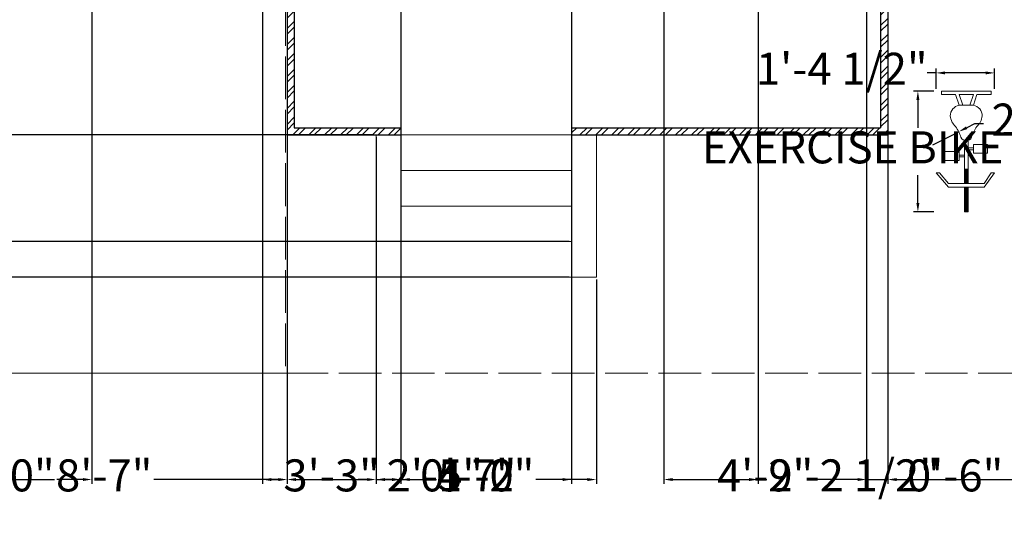
# Model space of a CAD drawing. Units: inches. Extents: x 9689 to 10369, y 10965 to 11626.
# Tile 2 of 11: x 9830 to 10107, y 10965 to 11108. Entities that reach past the tile are written whole.
import ezdxf

# ---------------------------------------------------------------- set-up
doc = ezdxf.new("R2010")
doc.units = ezdxf.units.IN
doc.linetypes.add('ACAD_ISO02W100', pattern=[15, 12, -3])
for name, color, linetype, lineweight in [('A-ANNO-DIMS', 2, 'Continuous', 18), ('A-EQPM', 8, 'Continuous', 18), ('A-FLOR', 7, 'Continuous', 25), ('A-FLOR-PATT', 252, 'Continuous', 13), ('A-FLOR-STRS', 7, 'Continuous', 18), ('C-PARK', 7, 'ACAD_ISO02W100', 18)]:
    doc.layers.add(name, color=color, linetype=linetype, lineweight=lineweight)
doc.styles.get("Standard").update_dxf_attribs({"font": 'arial.ttf'})
doc.dimstyles.new('ISO-25', dxfattribs={"dimtxt": 9, "dimasz": 2.5, "dimexe": 1.25, "dimexo": 0.625, "dimgap": 2, "dimtad": 0, "dimtih": 1, "dimtoh": 1, "dimdec": 1, "dimlunit": 4, "dimtxsty": 'Standard', "dimcen": 2.5, "dimadec": 0, "dimazin": 0, "dimtfac": 0.5, "dimtdec": 1, "dimtmove": 0, "dimatfit": 3, "dimfxl": 1, "dimarcsym": 0})

# ---------------------------------------------------------------- blocks, each defined once
blk = doc.blocks.new('Exercise Bike')
for p, q in [((-0.75, 10), (-0.75, 17)), ((-0.75, 17), (0.25, 17)), ((-0.5, 17), (-0.5, 9.9929)), ((-0.25, 10), (-0.25, 17)), ((0, 17), (0, 9.9929)), ((0.25, 17), (0.25, 10)), ((-5.25, 10), (-8.25, 6)), ((-7.25, 6), (-5.25, 9)), ((-0.75, 10), (-5.25, 10)), ((-5.25, 9), (4.75, 9)), ((4.75, 10), (-0.75, 10)), ((-0.75, 5), (-0.75, 9)), ((-0.5, 8.9396), (-0.5, 5)), ((-0.25, 5), (-0.25, 9)), ((0, 8.9396), (0, 5)), ((0.25, 9), (0.25, 5)), ((8.25, 6), (4.75, 10)), ((4.75, 9), (7.25, 6)), ((-8.25, 6), (-7.25, 6)), ((7.25, 6), (8.25, 6)), ((-0.75, -3.0635), (-0.75, 5)), ((-0.75, 5), (0.25, 5)), ((0.25, 5), (0.25, -3.0635)), ((-6.25, -2), (-6.25, 0.5)), ((-2.25, 0.5), (-6.25, 0.5)), ((-2.25, -0.5), (-2.25, 0.5)), ((0.25, 1.5), (1.75, 1.5)), ((0.25, 1), (1.75, 1)), ((1.75, 2.5), (5.75, 2.5)), ((1.75, 1.5), (1.75, 2.5)), ((1.75, 1.5), (1.75, 0)), ((1.75, 0), (5.75, 0)), ((5.75, 2.5), (5.75, 0)), ((-2.25, -2), (-6.25, -2)), ((-2.25, -0.5), (-0.75, -0.5)), ((-2.25, -1), (-2.25, -0.5)), ((-2.25, -1), (-2.25, -2)), ((-0.75, -1), (-2.25, -1)), ((-2.25, -13), (-3.25, -16)), ((-2.25, -16), (-1.25, -13)), ((-2.25, -13), (1.75, -13)), ((0.75, -13), (1.75, -16)), ((1.75, -13), (2.75, -16)), ((-7.25, -16), (-7.25, -17)), ((-4.75, -16), (-7.25, -16)), ((-3.25, -16), (-4.75, -16)), ((1.75, -16), (-2.25, -16)), ((6.75, -16), (2.75, -16)), ((6.75, -17), (6.75, -16)), ((-7.25, -17), (6.75, -17))]:
    blk.add_line(p, q)
for centre, radius, start, end in [((-9.6692, -1.9154), 8.1889, 321.6175, 345.2525), ((-0.25, -4.625), 1.625, 22.61987, 157.3801), ((9.1691, -1.9154), 8.1889, 194.7476, 218.3825), ((0.1685, -10.5843), 4.9531, 133.6443, 173.2256), ((-0.6686, -10.5843), 4.9531, 6.774486, 46.35562), ((-1.7006, -10.0005), 3.0494, 179.9906, 259.6205), ((1.2006, -10.0005), 3.0494, 280.3795, 0.009389)]:
    blk.add_arc(centre, radius, start, end)
blk = doc.blocks.new('*D62')
at = {"layer": 'A-ANNO-DIMS', "color": 0, "lineweight": -2, "transparency": 16777216}
for p, q in [((10087.02, 11087.95), (10081.3, 11087.95)), ((10082.55, 11085.45), (10082.55, 11077.6)), ((10082.55, 11056.45), (10082.55, 11064.29)), ((10087.02, 11053.95), (10081.3, 11053.95))]:
    blk.add_line(p, q, dxfattribs=at)
at = {"layer": 'A-ANNO-DIMS', "color": 0, "transparency": 16777216}
for points in [[(10082.13, 11085.45), (10082.96, 11085.45), (10082.55, 11087.95)], [(10082.13, 11056.45), (10082.96, 11056.45), (10082.55, 11053.95)]]:
    blk.add_solid(points, dxfattribs=at)
at = {"layer": 'Defpoints', "color": 0, "transparency": 16777216}
for p in [(10087.65, 11087.95), (10082.55, 11053.95), (10087.65, 11053.95)]:
    blk.add_point(p, dxfattribs=at)
at = {"layer": 'A-ANNO-DIMS', "color": 0, "transparency": 16777216, "insert": (10082.55, 11070.95), "char_height": 9, "attachment_point": 5}
blk.add_mtext('EXERCISE BIKE 2\'-10"', dxfattribs=at)
blk = doc.blocks.new('*D63')
at = {"layer": 'A-ANNO-DIMS', "color": 0, "lineweight": -2, "transparency": 16777216}
for p, q in [((10087.65, 11093.05), (10085.15, 11093.05)), ((10087.65, 11088.57), (10087.65, 11094.3)), ((10101.65, 11093.05), (10090.15, 11093.05)), ((10104.15, 11088.57), (10104.15, 11094.3))]:
    blk.add_line(p, q, dxfattribs=at)
at = {"layer": 'A-ANNO-DIMS', "color": 0, "transparency": 16777216}
for points in [[(10090.15, 11093.46), (10090.15, 11092.63), (10087.65, 11093.05)], [(10101.65, 11093.46), (10101.65, 11092.63), (10104.15, 11093.05)]]:
    blk.add_solid(points, dxfattribs=at)
at = {"layer": 'Defpoints', "color": 0, "transparency": 16777216}
for p in [(10087.65, 11093.05), (10087.65, 11087.95), (10104.15, 11087.95)]:
    blk.add_point(p, dxfattribs=at)
at = {"layer": 'A-ANNO-DIMS', "color": 0, "transparency": 16777216, "insert": (10061.12, 11093.05), "char_height": 9, "attachment_point": 5}
blk.add_mtext('1\'-4 1/2"', dxfattribs=at)
blk = doc.blocks.new('*D67')
at = {"layer": 'A-ANNO-DIMS', "color": 0, "lineweight": -2, "transparency": 16777216}
for p, q in [((9802.06, 11157.01), (9802.06, 10977.48)), ((9905.06, 11157.01), (9905.06, 10977.48)), ((9804.56, 10978.73), (9839.59, 10978.73)), ((9902.56, 10978.73), (9867.53, 10978.73))]:
    blk.add_line(p, q, dxfattribs=at)
at = {"layer": 'A-ANNO-DIMS', "color": 0, "transparency": 16777216}
for points in [[(9804.56, 10979.15), (9804.56, 10978.31), (9802.06, 10978.73)], [(9902.56, 10979.15), (9902.56, 10978.31), (9905.06, 10978.73)]]:
    blk.add_solid(points, dxfattribs=at)
at = {"layer": 'Defpoints', "color": 0, "transparency": 16777216}
for p in [(9802.06, 11157.63), (9905.06, 11157.63), (9905.06, 10978.73)]:
    blk.add_point(p, dxfattribs=at)
at = {"layer": 'A-ANNO-DIMS', "color": 0, "transparency": 16777216, "insert": (9853.56, 10978.73), "char_height": 9, "attachment_point": 5}
blk.add_mtext('8\'-7"', dxfattribs=at)
blk = doc.blocks.new('*D68')
at = {"layer": 'A-ANNO-DIMS', "color": 0, "lineweight": -2, "transparency": 16777216}
for p, q in [((9929.43, 11075.63), (9758.91, 11075.63)), ((9760.16, 11073.13), (9760.16, 11062.23)), ((9760.16, 11038.13), (9760.16, 11049.03)), ((9929.43, 11035.63), (9758.91, 11035.63))]:
    blk.add_line(p, q, dxfattribs=at)
at = {"layer": 'A-ANNO-DIMS', "color": 0, "transparency": 16777216}
for points in [[(9759.74, 11073.13), (9760.57, 11073.13), (9760.16, 11075.63)], [(9759.74, 11038.13), (9760.57, 11038.13), (9760.16, 11035.63)]]:
    blk.add_solid(points, dxfattribs=at)
at = {"layer": 'Defpoints', "color": 0, "transparency": 16777216}
for p in [(9760.16, 11075.63), (9930.06, 11075.63), (9930.06, 11035.63)]:
    blk.add_point(p, dxfattribs=at)
at = {"layer": 'A-ANNO-DIMS', "color": 0, "transparency": 16777216, "insert": (9760.16, 11055.63), "char_height": 9, "attachment_point": 5}
blk.add_mtext('3\'-4"', dxfattribs=at)
blk = doc.blocks.new('*D69')
at = {"layer": 'A-ANNO-DIMS', "color": 0, "lineweight": -2, "transparency": 16777216}
for p, q in [((9930.06, 11035.01), (9930.06, 10977.48)), ((9992.06, 11035.01), (9992.06, 10977.48)), ((9932.56, 10978.73), (9947.09, 10978.73)), ((9989.56, 10978.73), (9975.02, 10978.73))]:
    blk.add_line(p, q, dxfattribs=at)
at = {"layer": 'A-ANNO-DIMS', "color": 0, "transparency": 16777216}
for points in [[(9932.56, 10979.15), (9932.56, 10978.31), (9930.06, 10978.73)], [(9989.56, 10979.15), (9989.56, 10978.31), (9992.06, 10978.73)]]:
    blk.add_solid(points, dxfattribs=at)
at = {"layer": 'Defpoints', "color": 0, "transparency": 16777216}
for p in [(9930.06, 11035.63), (9992.06, 11035.63), (9992.06, 10978.73)]:
    blk.add_point(p, dxfattribs=at)
at = {"layer": 'A-ANNO-DIMS', "color": 0, "transparency": 16777216, "insert": (9961.06, 10978.73), "char_height": 9, "attachment_point": 5}
blk.add_mtext('5\'-2"', dxfattribs=at)
blk = doc.blocks.new('*D70')
at = {"layer": 'A-ANNO-DIMS', "color": 0, "lineweight": -2, "transparency": 16777216}
for p, q in [((10011.06, 11166.01), (10011.06, 10977.48)), ((10068.06, 11166.01), (10068.06, 10977.48)), ((10013.56, 10978.73), (10025.41, 10978.73)), ((10065.56, 10978.73), (10053.7, 10978.73))]:
    blk.add_line(p, q, dxfattribs=at)
at = {"layer": 'A-ANNO-DIMS', "color": 0, "transparency": 16777216}
for points in [[(10013.56, 10979.15), (10013.56, 10978.31), (10011.06, 10978.73)], [(10065.56, 10979.15), (10065.56, 10978.31), (10068.06, 10978.73)]]:
    blk.add_solid(points, dxfattribs=at)
at = {"layer": 'Defpoints', "color": 0, "transparency": 16777216}
for p in [(10011.06, 11166.63), (10068.06, 11166.63), (10068.06, 10978.73)]:
    blk.add_point(p, dxfattribs=at)
at = {"layer": 'A-ANNO-DIMS', "color": 0, "transparency": 16777216, "insert": (10039.56, 10978.73), "char_height": 9, "attachment_point": 5}
blk.add_mtext('4\'-9"', dxfattribs=at)
blk = doc.blocks.new('*D71')
at = {"layer": 'A-ANNO-DIMS', "color": 0, "lineweight": -2, "transparency": 16777216}
for p, q in [((10068.06, 11166.01), (10068.06, 10977.48)), ((10074.06, 11166.01), (10074.06, 10977.48)), ((10065.56, 10978.73), (10063.06, 10978.73)), ((10068.06, 10978.73), (10074.06, 10978.73)), ((10076.56, 10978.73), (10079.06, 10978.73))]:
    blk.add_line(p, q, dxfattribs=at)
at = {"layer": 'A-ANNO-DIMS', "color": 0, "transparency": 16777216}
for points in [[(10065.56, 10979.15), (10065.56, 10978.31), (10068.06, 10978.73)], [(10076.56, 10979.15), (10076.56, 10978.31), (10074.06, 10978.73)]]:
    blk.add_solid(points, dxfattribs=at)
at = {"layer": 'Defpoints', "color": 0, "transparency": 16777216}
for p in [(10068.06, 11166.63), (10074.06, 11166.63), (10074.06, 10978.73)]:
    blk.add_point(p, dxfattribs=at)
at = {"layer": 'A-ANNO-DIMS', "color": 0, "transparency": 16777216, "insert": (10093.02, 10978.73), "char_height": 9, "attachment_point": 5}
blk.add_mtext('0\'-6"', dxfattribs=at)
blk = doc.blocks.new('*D72')
at = {"layer": 'A-ANNO-DIMS', "color": 0, "lineweight": -2, "transparency": 16777216}
for p, q in [((10011.06, 11211.16), (10011.06, 10977.48)), ((10037.56, 11211.16), (10037.56, 10977.48)), ((10013.56, 10978.73), (10035.06, 10978.73)), ((10037.56, 10978.73), (10040.06, 10978.73))]:
    blk.add_line(p, q, dxfattribs=at)
at = {"layer": 'A-ANNO-DIMS', "color": 0, "transparency": 16777216}
for points in [[(10013.56, 10979.15), (10013.56, 10978.31), (10011.06, 10978.73)], [(10035.06, 10979.15), (10035.06, 10978.31), (10037.56, 10978.73)]]:
    blk.add_solid(points, dxfattribs=at)
at = {"layer": 'Defpoints', "color": 0, "transparency": 16777216}
for p in [(10011.06, 11211.79), (10037.56, 11211.79), (10037.56, 10978.73)]:
    blk.add_point(p, dxfattribs=at)
at = {"layer": 'A-ANNO-DIMS', "color": 0, "transparency": 16777216, "insert": (10064.58, 10978.73), "char_height": 9, "attachment_point": 5}
blk.add_mtext('2\'-2 1/2"', dxfattribs=at)
blk = doc.blocks.new('*D85')
at = {"layer": 'A-ANNO-DIMS', "color": 0, "lineweight": -2, "transparency": 16777216}
for p, q in [((9937.06, 11157.01), (9937.06, 10977.48)), ((9985.06, 11157.01), (9985.06, 10977.48)), ((9939.56, 10978.73), (9946.91, 10978.73)), ((9982.56, 10978.73), (9975.2, 10978.73))]:
    blk.add_line(p, q, dxfattribs=at)
at = {"layer": 'A-ANNO-DIMS', "color": 0, "transparency": 16777216}
for points in [[(9939.56, 10979.15), (9939.56, 10978.31), (9937.06, 10978.73)], [(9982.56, 10979.15), (9982.56, 10978.31), (9985.06, 10978.73)]]:
    blk.add_solid(points, dxfattribs=at)
at = {"layer": 'Defpoints', "color": 0, "transparency": 16777216}
for p in [(9937.06, 11157.63), (9985.06, 11157.63), (9985.06, 10978.73)]:
    blk.add_point(p, dxfattribs=at)
at = {"layer": 'A-ANNO-DIMS', "color": 0, "transparency": 16777216, "insert": (9961.06, 10978.73), "char_height": 9, "attachment_point": 5}
blk.add_mtext('4\'-0"', dxfattribs=at)
blk = doc.blocks.new('*D87')
at = {"layer": 'A-ANNO-DIMS', "color": 0, "lineweight": -2, "transparency": 16777216}
for p, q in [((9802.06, 11157.01), (9802.06, 10977.48)), ((9850.06, 11157.01), (9850.06, 10977.48)), ((9804.56, 10978.73), (9811.91, 10978.73)), ((9847.56, 10978.73), (9840.2, 10978.73))]:
    blk.add_line(p, q, dxfattribs=at)
at = {"layer": 'A-ANNO-DIMS', "color": 0, "transparency": 16777216}
for points in [[(9804.56, 10979.15), (9804.56, 10978.31), (9802.06, 10978.73)], [(9847.56, 10979.15), (9847.56, 10978.31), (9850.06, 10978.73)]]:
    blk.add_solid(points, dxfattribs=at)
at = {"layer": 'Defpoints', "color": 0, "transparency": 16777216}
for p in [(9802.06, 11157.63), (9850.06, 11157.63), (9850.06, 10978.73)]:
    blk.add_point(p, dxfattribs=at)
at = {"layer": 'A-ANNO-DIMS', "color": 0, "transparency": 16777216, "insert": (9826.06, 10978.73), "char_height": 9, "attachment_point": 5}
blk.add_mtext('4\'-0"', dxfattribs=at)
blk = doc.blocks.new('*D88')
at = {"layer": 'A-ANNO-DIMS', "color": 0, "lineweight": -2, "transparency": 16777216}
for p, q in [((9898.06, 11157.01), (9898.06, 10977.48)), ((9937.06, 11157.01), (9937.06, 10977.48)), ((9900.56, 10978.73), (9903.6, 10978.73)), ((9934.56, 10978.73), (9931.52, 10978.73))]:
    blk.add_line(p, q, dxfattribs=at)
at = {"layer": 'A-ANNO-DIMS', "color": 0, "transparency": 16777216}
for points in [[(9900.56, 10979.15), (9900.56, 10978.31), (9898.06, 10978.73)], [(9934.56, 10979.15), (9934.56, 10978.31), (9937.06, 10978.73)]]:
    blk.add_solid(points, dxfattribs=at)
at = {"layer": 'Defpoints', "color": 0, "transparency": 16777216}
for p in [(9898.06, 11157.63), (9937.06, 11157.63), (9937.06, 10978.73)]:
    blk.add_point(p, dxfattribs=at)
at = {"layer": 'A-ANNO-DIMS', "color": 0, "transparency": 16777216, "insert": (9917.56, 10978.73), "char_height": 9, "attachment_point": 5}
blk.add_mtext('3\'-3"', dxfattribs=at)
blk = doc.blocks.new('*D95')
at = {"layer": 'A-ANNO-DIMS', "color": 0, "lineweight": -2, "transparency": 16777216}
for p, q in [((9905.06, 11075.01), (9905.06, 10977.48)), ((9930.06, 11075.01), (9930.06, 10977.48)), ((9907.56, 10978.73), (9927.56, 10978.73)), ((9930.06, 10978.73), (9932.56, 10978.73))]:
    blk.add_line(p, q, dxfattribs=at)
at = {"layer": 'A-ANNO-DIMS', "color": 0, "transparency": 16777216}
for points in [[(9907.56, 10979.15), (9907.56, 10978.31), (9905.06, 10978.73)], [(9927.56, 10979.15), (9927.56, 10978.31), (9930.06, 10978.73)]]:
    blk.add_solid(points, dxfattribs=at)
at = {"layer": 'Defpoints', "color": 0, "transparency": 16777216}
for p in [(9905.06, 11075.63), (9930.06, 11075.63), (9930.06, 10978.73)]:
    blk.add_point(p, dxfattribs=at)
at = {"layer": 'A-ANNO-DIMS', "color": 0, "transparency": 16777216, "insert": (9946.6, 10978.73), "char_height": 9, "attachment_point": 5}
blk.add_mtext('2\'-1"', dxfattribs=at)
blk = doc.blocks.new('*D96')
at = {"layer": 'A-ANNO-DIMS', "color": 0, "lineweight": -2, "transparency": 16777216}
for p, q in [((10074.06, 11075.01), (10074.06, 10977.48)), ((10244.06, 11008.01), (10244.06, 10977.48)), ((10076.56, 10978.73), (10142.02, 10978.73)), ((10241.56, 10978.73), (10176.09, 10978.73))]:
    blk.add_line(p, q, dxfattribs=at)
at = {"layer": 'A-ANNO-DIMS', "color": 0, "transparency": 16777216}
for points in [[(10076.56, 10979.15), (10076.56, 10978.31), (10074.06, 10978.73)], [(10241.56, 10979.15), (10241.56, 10978.31), (10244.06, 10978.73)]]:
    blk.add_solid(points, dxfattribs=at)
at = {"layer": 'Defpoints', "color": 0, "transparency": 16777216}
for p in [(10074.06, 11075.63), (10244.06, 11008.63), (10244.06, 10978.73)]:
    blk.add_point(p, dxfattribs=at)
at = {"layer": 'A-ANNO-DIMS', "color": 0, "transparency": 16777216, "insert": (10159.06, 10978.73), "char_height": 9, "attachment_point": 5}
blk.add_mtext('14\'-2"', dxfattribs=at)
blk = doc.blocks.new('*D112')
at = {"layer": 'A-ANNO-DIMS', "color": 0, "lineweight": -2, "transparency": 16777216}
for p, q in [((9930.06, 11035.01), (9930.06, 10977.48)), ((9937.06, 11035.01), (9937.06, 10977.48)), ((9927.56, 10978.73), (9925.06, 10978.73)), ((9930.06, 10978.73), (9937.06, 10978.73)), ((9939.56, 10978.73), (9942.06, 10978.73))]:
    blk.add_line(p, q, dxfattribs=at)
at = {"layer": 'A-ANNO-DIMS', "color": 0, "transparency": 16777216}
for points in [[(9927.56, 10979.15), (9927.56, 10978.31), (9930.06, 10978.73)], [(9939.56, 10979.15), (9939.56, 10978.31), (9937.06, 10978.73)]]:
    blk.add_solid(points, dxfattribs=at)
at = {"layer": 'Defpoints', "color": 0, "transparency": 16777216}
for p in [(9930.06, 11035.63), (9937.06, 11035.63), (9937.06, 10978.73)]:
    blk.add_point(p, dxfattribs=at)
at = {"layer": 'A-ANNO-DIMS', "color": 0, "transparency": 16777216, "insert": (9956.02, 10978.73), "char_height": 9, "attachment_point": 5}
blk.add_mtext('0\'-7"', dxfattribs=at)
blk = doc.blocks.new('*D113')
at = {"layer": 'A-ANNO-DIMS', "color": 0, "lineweight": -2, "transparency": 16777216}
for p, q in [((9760.16, 11045.63), (9760.16, 11048.13)), ((9760.16, 11048.13), (9762.66, 11048.13)), ((9984.43, 11045.63), (9758.91, 11045.63)), ((9760.16, 11038.13), (9760.16, 11043.13)), ((9984.43, 11035.63), (9758.91, 11035.63))]:
    blk.add_line(p, q, dxfattribs=at)
at = {"layer": 'A-ANNO-DIMS', "color": 0, "transparency": 16777216}
for points in [[(9759.74, 11043.13), (9760.57, 11043.13), (9760.16, 11045.63)], [(9759.74, 11038.13), (9760.57, 11038.13), (9760.16, 11035.63)]]:
    blk.add_solid(points, dxfattribs=at)
at = {"layer": 'Defpoints', "color": 0, "transparency": 16777216}
for p in [(9760.16, 11045.63), (9985.06, 11045.63), (9985.06, 11035.63)]:
    blk.add_point(p, dxfattribs=at)
at = {"layer": 'A-ANNO-DIMS', "color": 0, "transparency": 16777216, "insert": (9780.12, 11048.13), "char_height": 9, "attachment_point": 5}
blk.add_mtext('0\'-10"', dxfattribs=at)
blk = doc.blocks.new('*D130')
at = {"layer": 'A-ANNO-DIMS', "color": 0, "lineweight": -2, "transparency": 16777216}
for p, q in [((10098.52, 11078.76), (10096.29, 11077.64)), ((10101.02, 11078.76), (10098.52, 11078.76)), ((10086.73, 11072.86), (10094.05, 11076.52))]:
    blk.add_line(p, q, dxfattribs=at)
at = {"layer": 'A-ANNO-DIMS', "color": 0, "transparency": 16777216}
blk.add_solid([(10096.1, 11078.02), (10096.47, 11077.27), (10094.05, 11076.52)], dxfattribs=at)
at = {"layer": 'Defpoints', "color": 0, "transparency": 16777216}
for p in [(10094.05, 11076.52), (10086.73, 11072.86)]:
    blk.add_point(p, dxfattribs=at)
at = {"layer": 'A-ANNO-DIMS', "color": 0, "transparency": 16777216, "insert": (10129.04, 11078.76), "char_height": 9, "attachment_point": 5}
blk.add_mtext('2X R0\'-8"', dxfattribs=at)

msp = doc.modelspace()

# ---------------------------------------------------------------- hatches: boundary and pattern name
at = {"layer": 'A-FLOR-PATT'}
h = msp.add_hatch(dxfattribs=at)
h.set_pattern_fill('STEEL', color=256)
h.set_pattern_definition([(45, (0, 0), (-2.245064, 2.245064), []), (45, (0, 1.5875), (-2.245064, 2.245064), [])])
h.paths.add_polyline_path([(10074.06, 11157.63), (10072.06, 11157.63), (10072.06, 11077.63), (9985.06, 11077.63), (9985.06, 11075.63), (10074.06, 11075.63)])
h.paths.add_polyline_path([(9907.06, 11157.63), (9905.06, 11157.63), (9905.06, 11075.63), (9937.06, 11075.63), (9937.06, 11077.63), (9907.06, 11077.63)])

# ---------------------------------------------------------------- linework, layer by layer
at = {"layer": 'A-ANNO-DIMS'}
msp.add_line((9904.55, 11008.63), (9802.06, 11008.63), dxfattribs=at)
at = {"layer": 'A-FLOR'}
for p, q in [((9905.06, 11157.63), (9905.06, 11075.63)), ((9907.06, 11157.63), (9907.06, 11077.63)), ((10072.06, 11157.63), (10072.06, 11077.63)), ((10074.06, 11157.63), (10074.06, 11075.63)), ((9905.06, 11075.63), (9937.06, 11075.63)), ((9907.06, 11077.63), (9937.06, 11077.63)), ((9937.06, 11077.63), (9937.06, 11075.63)), ((9985.06, 11077.63), (9985.06, 11075.63)), ((9985.06, 11077.63), (10072.06, 11077.63)), ((9985.06, 11075.63), (10074.06, 11075.63))]:
    msp.add_line(p, q, dxfattribs=at)
at = {"layer": 'A-FLOR-STRS'}
for p, q in [((9930.06, 11075.63), (9930.06, 11035.63)), ((9937.06, 11075.63), (9985.06, 11075.63)), ((9937.06, 11075.63), (9937.06, 11035.63)), ((9985.06, 11075.63), (9985.06, 11035.63)), ((9992.06, 11075.63), (9992.06, 11035.63)), ((9937.06, 11065.63), (9985.06, 11065.63)), ((9937.06, 11055.63), (9985.06, 11055.63)), ((9937.06, 11045.63), (9985.06, 11045.63)), ((9930.06, 11035.63), (9992.06, 11035.63)), ((9937.06, 11035.63), (9985.06, 11035.63))]:
    msp.add_line(p, q, dxfattribs=at)
at = {"layer": 'C-PARK'}
for p, q in [((9904.55, 11157.63), (9904.55, 11008.63)), ((9904.55, 11008.63), (10244.06, 11008.63))]:
    msp.add_line(p, q, dxfattribs=at)

# ---------------------------------------------------------------- block references
at = {"layer": 'A-EQPM', "rotation": 180}
msp.add_blockref('Exercise Bike', (10095.9, 11070.95), dxfattribs=at)

# ---------------------------------------------------------------- dimensions: what is measured, and where the dimension line sits
at = {"layer": 'A-ANNO-DIMS'}
for base, p1, p2, picture, middle in [((10037.56, 10978.73), (10011.06, 11211.79), (10037.56, 11211.79), '*D72', (10064.58, 10978.73)), ((10068.06, 10978.73), (10011.06, 11166.63), (10068.06, 11166.63), '*D70', (10039.56, 10978.73)), ((10074.06, 10978.73), (10068.06, 11166.63), (10074.06, 11166.63), '*D71', (10093.02, 10978.73)), ((9905.06, 10978.73), (9802.06, 11157.63), (9905.06, 11157.63), '*D67', (9853.56, 10978.73)), ((9850.06, 10978.73), (9802.06, 11157.63), (9850.06, 11157.63), '*D87', (9826.06, 10978.73)), ((9937.06, 10978.73), (9898.06, 11157.63), (9937.06, 11157.63), '*D88', (9917.56, 10978.73)), ((9985.06, 10978.73), (9937.06, 11157.63), (9985.06, 11157.63), '*D85', (9961.06, 10978.73)), ((9930.06, 10978.73), (9905.06, 11075.63), (9930.06, 11075.63), '*D95', (9946.6, 10978.73)), ((10244.06, 10978.73), (10074.06, 11075.63), (10244.06, 11008.63), '*D96', (10159.06, 10978.73)), ((9937.06, 10978.73), (9930.06, 11035.63), (9937.06, 11035.63), '*D112', (9956.02, 10978.73)), ((9992.06, 10978.73), (9930.06, 11035.63), (9992.06, 11035.63), '*D69', (9961.06, 10978.73))]:
    dim = msp.add_linear_dim(base=base, p1=p1, p2=p2, dimstyle='ISO-25', override={"dimdec": 1, "dimlfac": 1, "dimrnd": 0, "dimzin": 1, "dimdsep": 46, "dimlunit": 4, "dimfrac": 2}, dxfattribs=at)
    dim.commit()
    dim.dimension.update_dxf_attribs({"geometry": picture, "text_midpoint": middle})
for base, p1, p2, angle, picture, middle in [((10087.65, 11093.05), (10104.15, 11087.95), (10087.65, 11087.95), 180, '*D63', (10061.12, 11093.05)), ((9760.16, 11075.63), (9930.06, 11035.63), (9930.06, 11075.63), 90, '*D68', (9760.16, 11055.63)), ((9760.16, 11045.63), (9985.06, 11035.63), (9985.06, 11045.63), 90, '*D113', (9780.12, 11048.13))]:
    dim = msp.add_linear_dim(base=base, p1=p1, p2=p2, angle=angle, dimstyle='ISO-25', override={"dimdec": 1, "dimlfac": 1, "dimrnd": 0, "dimzin": 1, "dimdsep": 46, "dimlunit": 4, "dimfrac": 2}, dxfattribs=at)
    dim.commit()
    dim.dimension.update_dxf_attribs({"geometry": picture, "text_midpoint": middle})
dim = msp.add_radius_dim(center=(10086.73, 11072.86), mpoint=(10094.05, 11076.52), text='2X <>', dimstyle='ISO-25', override={"dimdec": 1, "dimlfac": 1, "dimrnd": 0, "dimzin": 1, "dimdsep": 46, "dimlunit": 4, "dimfrac": 2}, dxfattribs=at)
dim.commit()
dim.dimension.update_dxf_attribs({"geometry": '*D130', "text_midpoint": (10129.04, 11078.76)})
dim = msp.add_linear_dim(base=(10082.55, 11053.95), p1=(10087.65, 11087.95), p2=(10087.65, 11053.95), angle=270, text='EXERCISE BIKE <>', dimstyle='ISO-25', override={"dimdec": 1, "dimlfac": 1, "dimrnd": 0, "dimzin": 1, "dimdsep": 46, "dimlunit": 4, "dimfrac": 2}, dxfattribs=at)
dim.commit()
dim.dimension.update_dxf_attribs({"geometry": '*D62', "text_midpoint": (10082.55, 11070.95)})

doc.saveas('drawing.dxf')
